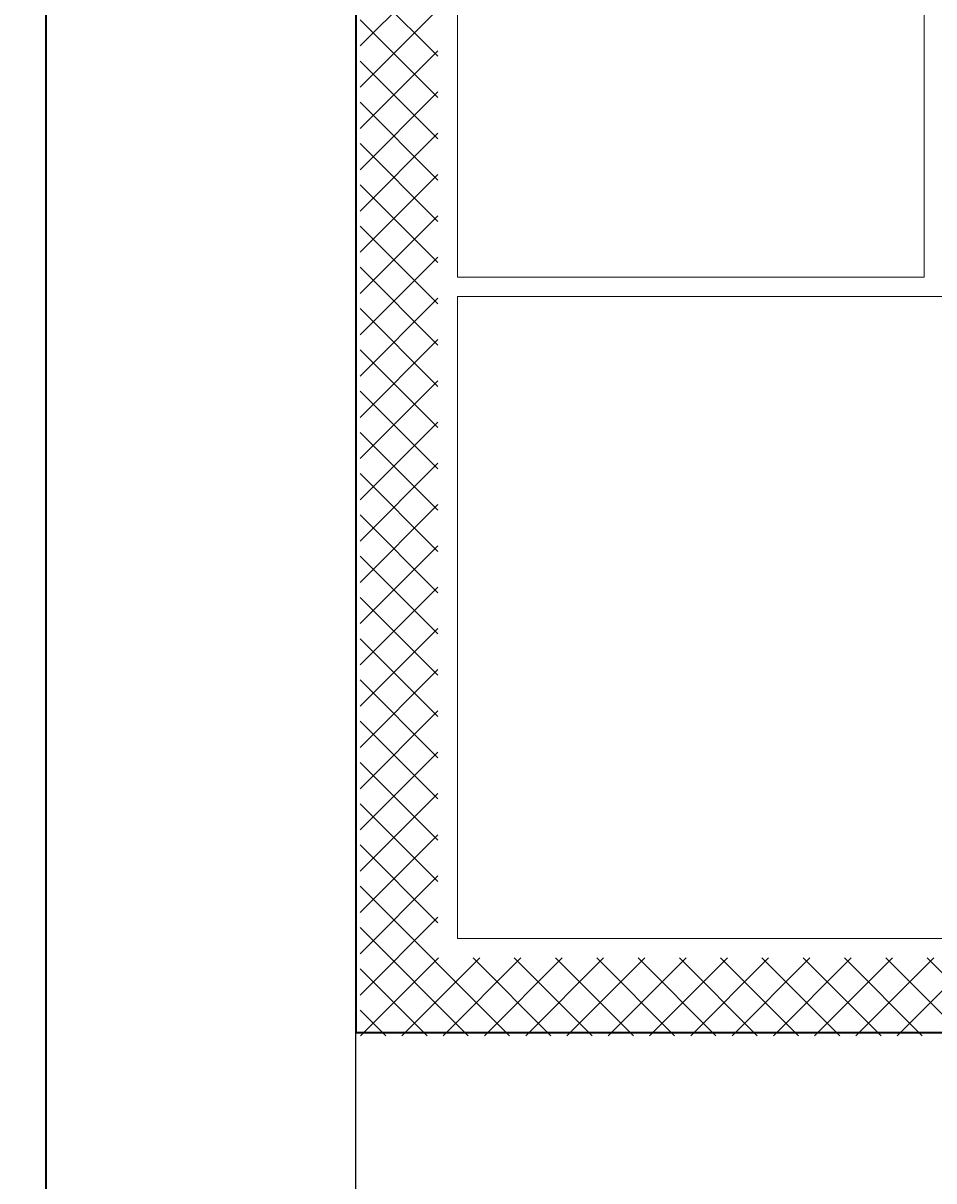
# Model space of a CAD drawing. Units: inches. Extents: x 4159 to 4826, y 299 to 1026.
# Tile 13 of 37: x 4192 to 4218, y 596 to 630. Entities that reach past the tile are written whole.
import ezdxf

# ---------------------------------------------------------------- set-up
doc = ezdxf.new("R2010")
doc.units = ezdxf.units.IN
for name, color, linetype, lineweight in [('A-ANNO-DIMS', 2, 'Continuous', 18), ('A-FLOR-FIXT', 9, 'Continuous', 18), ('A-WALL', 7, 'Continuous', 35)]:
    doc.layers.add(name, color=color, linetype=linetype, lineweight=lineweight)
doc.styles.get("Standard").update_dxf_attribs({"font": 'arial.ttf'})
doc.dimstyles.get("Standard").update_dxf_attribs({"dimtxt": 0.18, "dimasz": 0.18, "dimexe": 0.18, "dimexo": 0.0625, "dimgap": 0.09, "dimtad": 0, "dimtih": 1, "dimtoh": 1, "dimdec": 4, "dimzin": 0, "dimdsep": 46, "dimtxsty": 'Standard', "dimcen": 0.09, "dimadec": 0, "dimazin": 0, "dimtfac": 1, "dimtdec": 4, "dimtofl": 0, "dimtmove": 0, "dimatfit": 3, "dimfxl": 1, "dimtolj": 1, "dimtzin": 0, "dimarcsym": 0})

# ---------------------------------------------------------------- blocks, each defined once
blk = doc.blocks.new('Kitchen Layout - 7 x 8 ft')
for p, q in [((-5, 81.316), (2.684, 89)), ((-5, 83.437), (0.563, 89)), ((-5, 85.558), (-1.558, 89)), ((-5, 87.68), (-3.68, 89)), ((-1, 84.971), (-5, 88.971)), ((1.093, 85), (-2.907, 89)), ((3.214, 85), (-0.786, 89)), ((0.806, 85), (4.806, 89)), ((5.335, 85), (1.335, 89)), ((2.927, 85), (6.927, 89)), ((7.457, 85), (3.457, 89)), ((5.048, 85), (9.048, 89)), ((9.578, 85), (5.578, 89)), ((7.17, 85), (11.17, 89)), ((11.699, 85), (7.699, 89)), ((9.291, 85), (13.291, 89)), ((13.821, 85), (9.821, 89)), ((11.412, 85), (15.412, 89)), ((15.942, 85), (11.942, 89)), ((13.534, 85), (17.534, 89)), ((18.063, 85), (14.063, 89)), ((15.655, 85), (19.655, 89)), ((20.185, 85), (16.185, 89)), ((17.776, 85), (21.776, 89)), ((22.306, 85), (18.306, 89)), ((19.898, 85), (23.898, 89)), ((24.427, 85), (20.427, 89)), ((22.019, 85), (26.019, 89)), ((26.549, 85), (22.549, 89)), ((24.14, 85), (28.14, 89)), ((28.67, 85), (24.67, 89)), ((26.261, 85), (30.261, 89)), ((30.791, 85), (26.791, 89)), ((28.383, 85), (32.383, 89)), ((32.913, 85), (28.913, 89)), ((30.504, 85), (34.504, 89)), ((35.034, 85), (31.034, 89)), ((32.625, 85), (36.625, 89)), ((37.155, 85), (33.155, 89)), ((34.747, 85), (38.747, 89)), ((39.276, 85), (35.276, 89)), ((36.868, 85), (40.868, 89)), ((41.398, 85), (37.398, 89)), ((38.989, 85), (42.989, 89)), ((43.519, 85), (39.519, 89)), ((41.111, 85), (45.111, 89)), ((45.64, 85), (41.64, 89)), ((43.232, 85), (47.232, 89)), ((47.762, 85), (43.762, 89)), ((45.353, 85), (49.353, 89)), ((49.883, 85), (45.883, 89)), ((-1, 82.85), (-5, 86.85)), ((-1, 80.729), (-5, 84.729)), ((34, 84), (96, 84)), ((34, 60), (34, 84)), ((-5, 79.194), (-1, 83.194)), ((-1, 78.607), (-5, 82.607)), ((-5, 77.073), (-1, 81.073)), ((-1, 76.486), (-5, 80.486)), ((-5, 74.952), (-1, 78.952)), ((-1, 74.365), (-5, 78.365)), ((-5, 72.83), (-1, 76.83)), ((-1, 72.243), (-5, 76.243)), ((-5, 70.709), (-1, 74.709)), ((-1, 70.122), (-5, 74.122)), ((-5, 68.588), (-1, 72.588)), ((-1, 68.001), (-5, 72.001)), ((-5, 66.466), (-1, 70.466)), ((-1, 65.88), (-5, 69.88)), ((-5, 64.345), (-1, 68.345)), ((-1, 63.758), (-5, 67.758)), ((-5, 62.224), (-1, 66.224)), ((-1, 61.637), (-5, 65.637)), ((-5, 60.102), (-1, 64.102)), ((-1, 59.516), (-5, 63.516)), ((-5, 57.981), (-1, 61.981)), ((-1, 57.394), (-5, 61.394)), ((-4.86, 56), (-1, 59.86)), ((96, 60), (34, 60))]:
    blk.add_line(p, q)
blk.add_lwpolyline([(0, 56), (0, 84), (33, 84), (33, 56)], close=True)
blk = doc.blocks.new('*D44')
at = {"layer": 'A-ANNO-DIMS', "color": 0, "lineweight": -2, "transparency": 16777216}
for p, q in [((4287.263, 963.093), (4158.88, 963.093)), ((4159.06, 962.913), (4159.06, 647.826)), ((4159.06, 332.375), (4159.06, 647.462)), ((4447.248, 332.195), (4158.88, 332.195))]:
    blk.add_line(p, q, dxfattribs=at)
at = {"layer": 'A-ANNO-DIMS', "color": 0, "transparency": 16777216}
for points in [[(4159.03, 962.913), (4159.09, 962.913), (4159.06, 963.093)], [(4159.03, 332.375), (4159.09, 332.375), (4159.06, 332.195)]]:
    blk.add_solid(points, dxfattribs=at)
at = {"layer": 'Defpoints', "color": 0, "transparency": 16777216}
for p in [(4287.326, 963.093), (4159.06, 332.195), (4447.31, 332.195)]:
    blk.add_point(p, dxfattribs=at)
at = {"layer": 'A-ANNO-DIMS', "color": 0, "transparency": 16777216, "insert": (4159.06, 647.644), "char_height": 0.18, "attachment_point": 5}
blk.add_mtext('\\A1;630.9', dxfattribs=at)
blk = doc.blocks.new('*D50')
at = {"layer": 'A-ANNO-DIMS', "color": 0, "lineweight": -2, "transparency": 16777216}
for p, q in [((4192.31, 392.317), (4192.31, 1025.842)), ((4201.31, 401.317), (4201.31, 1025.842)), ((4192.49, 1025.662), (4196.661, 1025.662)), ((4201.13, 1025.662), (4196.959, 1025.662))]:
    blk.add_line(p, q, dxfattribs=at)
at = {"layer": 'A-ANNO-DIMS', "color": 0, "transparency": 16777216}
for points in [[(4192.49, 1025.692), (4192.49, 1025.632), (4192.31, 1025.662)], [(4201.13, 1025.692), (4201.13, 1025.632), (4201.31, 1025.662)]]:
    blk.add_solid(points, dxfattribs=at)
at = {"layer": 'Defpoints', "color": 0, "transparency": 16777216}
for p in [(4201.31, 1025.662), (4201.31, 401.254), (4192.31, 392.254)]:
    blk.add_point(p, dxfattribs=at)
at = {"layer": 'A-ANNO-DIMS', "color": 0, "transparency": 16777216, "insert": (4196.81, 1025.662), "char_height": 0.18, "attachment_point": 5}
blk.add_mtext('\\A1;9', dxfattribs=at)
blk = doc.blocks.new('*D51')
at = {"layer": 'A-ANNO-DIMS', "color": 0, "lineweight": -2, "transparency": 16777216}
for p, q in [((4201.248, 660.254), (4158.88, 660.254)), ((4159.06, 660.074), (4159.06, 526.436)), ((4159.06, 392.434), (4159.06, 526.072)), ((4192.248, 392.254), (4158.88, 392.254))]:
    blk.add_line(p, q, dxfattribs=at)
at = {"layer": 'A-ANNO-DIMS', "color": 0, "transparency": 16777216}
for points in [[(4159.03, 660.074), (4159.09, 660.074), (4159.06, 660.254)], [(4159.03, 392.434), (4159.09, 392.434), (4159.06, 392.254)]]:
    blk.add_solid(points, dxfattribs=at)
at = {"layer": 'Defpoints', "color": 0, "transparency": 16777216}
for p in [(4159.06, 660.254), (4201.31, 660.254), (4192.31, 392.254)]:
    blk.add_point(p, dxfattribs=at)
at = {"layer": 'A-ANNO-DIMS', "color": 0, "transparency": 16777216, "insert": (4159.06, 526.254), "char_height": 0.18, "attachment_point": 5}
blk.add_mtext('\\A1;268', dxfattribs=at)

msp = doc.modelspace()

# ---------------------------------------------------------------- linework, layer by layer
at = {"layer": 'A-WALL'}
for p in [(4201.31, 660.254), (4277.31, 600.254)]:
    msp.add_line(p, (4201.31, 600.254), dxfattribs=at)
msp.add_lwpolyline([(4303.31, 903.254), (4192.31, 903.254), (4192.31, 392.254)], dxfattribs=at)

# ---------------------------------------------------------------- block references
at = {"layer": 'A-FLOR-FIXT', "xscale": 0.5650329326971529, "yscale": 0.5650329326971529, "zscale": 0.5650329326971529, "rotation": 90}
msp.add_blockref('Kitchen Layout - 7 x 8 ft', (4251.725, 602.991), dxfattribs=at)

# ---------------------------------------------------------------- dimensions: what is measured, and where the dimension line sits
at = {"layer": 'A-ANNO-DIMS'}
dim = msp.add_linear_dim(base=(4201.31, 1025.662), p1=(4192.31, 392.254), p2=(4201.31, 401.254), dimstyle='Standard', override={"dimdec": 0, "dimlfac": 1, "dimrnd": 0, "dimzin": 0, "dimdsep": 46, "dimlunit": 2}, dxfattribs=at)
dim.commit()
dim.dimension.update_dxf_attribs({"geometry": '*D50', "text_midpoint": (4196.81, 1025.662)})
for base, p1, p2, override, picture, middle in [((4159.06, 332.195), (4287.326, 963.093), (4447.31, 332.195), {"dimdec": 1, "dimlfac": 1, "dimrnd": 0, "dimzin": 0, "dimdsep": 46, "dimlunit": 2}, '*D44', (4159.06, 647.644)), ((4159.06, 660.254), (4192.31, 392.254), (4201.31, 660.254), {"dimdec": 0, "dimlfac": 1, "dimrnd": 0, "dimzin": 0, "dimdsep": 46, "dimlunit": 2}, '*D51', (4159.06, 526.254))]:
    dim = msp.add_linear_dim(base=base, p1=p1, p2=p2, angle=90, dimstyle='Standard', override=override, dxfattribs=at)
    dim.commit()
    dim.dimension.update_dxf_attribs({"geometry": picture, "text_midpoint": middle})

doc.saveas('drawing.dxf')
